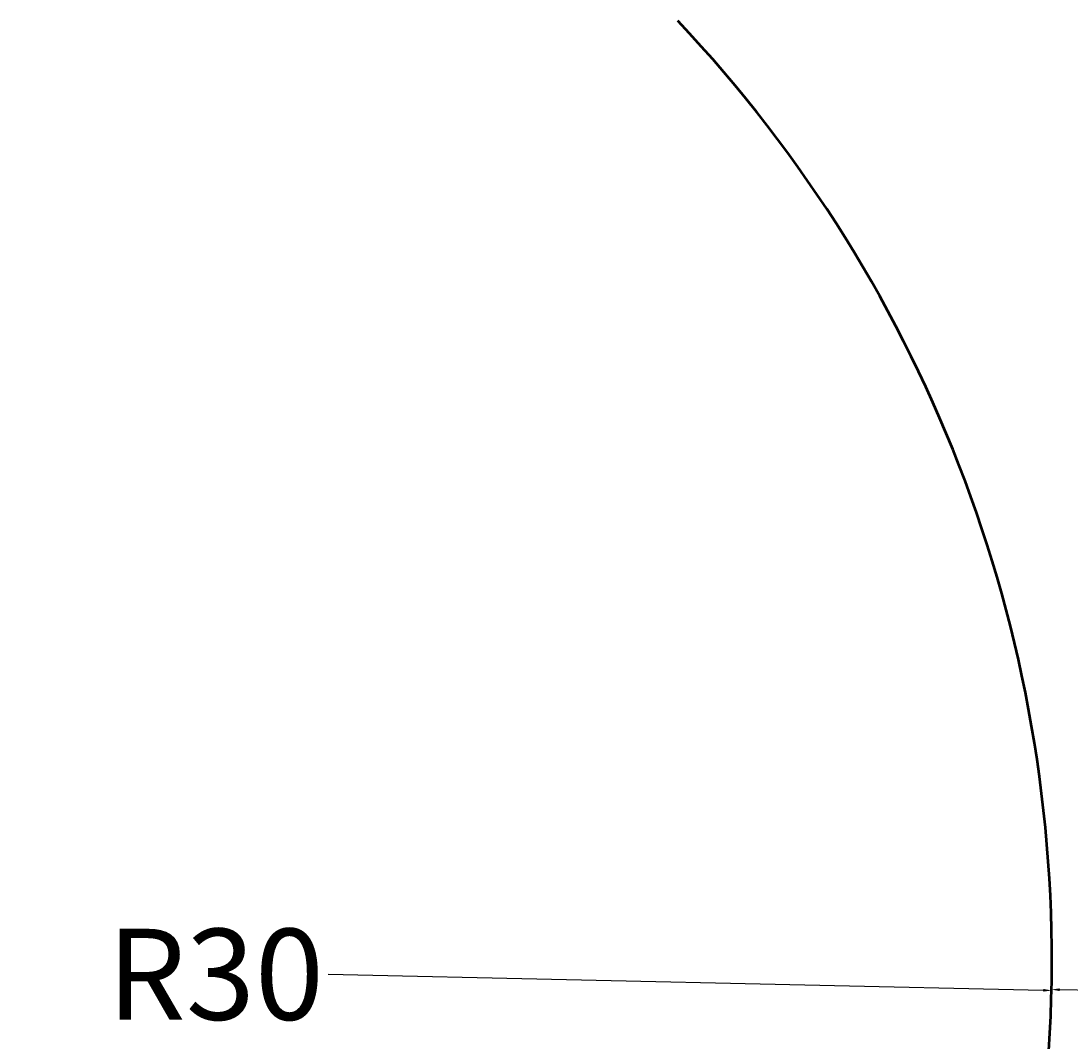
# Model space of a CAD drawing. Units: millimetres. Extents: x -60 to 113, y -37 to 126.
# Tile 8 of 17: x -23 to 0, y 48 to 70. Entities that reach past the tile are written whole.
import ezdxf

# ---------------------------------------------------------------- set-up
doc = ezdxf.new("R2010")
doc.units = ezdxf.units.MM
doc.header["$MEASUREMENT"] = 0
doc.layers.add('M-DIMS', color=2, linetype='Continuous', lineweight=25)
doc.layers.add('M-OUTL', color=7, linetype='Continuous', lineweight=50)
doc.styles.get("Standard").update_dxf_attribs({"font": 'arial.ttf'})
doc.dimstyles.get("Standard").update_dxf_attribs({"dimtxt": 0.18, "dimasz": 0.18, "dimexe": 0.18, "dimexo": 0.0625, "dimgap": 0.09, "dimtad": 0, "dimtih": 1, "dimtoh": 1, "dimdec": 4, "dimzin": 0, "dimdsep": 46, "dimtxsty": 'Standard', "dimcen": 0.09, "dimadec": 0, "dimazin": 0, "dimtfac": 1, "dimtdec": 4, "dimtofl": 0, "dimtmove": 0, "dimatfit": 3, "dimfxl": 1, "dimtolj": 1, "dimtzin": 0, "dimarcsym": 0})

# ---------------------------------------------------------------- blocks, each defined once
blk = doc.blocks.new('*D6')
at = {"layer": 'Defpoints', "color": 0, "transparency": 16777216}
for p in [(-30.775, 49.351), (-0.783, 48.68)]:
    blk.add_point(p, dxfattribs=at)
at = {"layer": 'M-DIMS', "color": 0, "lineweight": -2, "transparency": 16777216}
blk.add_line((-16.661, 49.035), (-0.963, 48.684), dxfattribs=at)
at = {"layer": 'M-DIMS', "color": 0, "transparency": 16777216}
blk.add_solid([(-0.962, 48.714), (-0.963, 48.654), (-0.783, 48.68)], dxfattribs=at)
at = {"layer": 'M-DIMS', "color": 0, "transparency": 16777216, "insert": (-19.137, 49.035), "char_height": 0.18, "attachment_point": 5}
blk.add_mtext('\\A1;{\\H11.11111x;R30}', dxfattribs=at)
blk = doc.blocks.new('*D7')
at = {"layer": 'Defpoints', "color": 0, "transparency": 16777216}
for p in [(48.606, 76.822), (-30.775, 49.351)]:
    blk.add_point(p, dxfattribs=at)
at = {"layer": 'M-DIMS', "color": 0, "lineweight": -2, "transparency": 16777216}
for p, q in [((37.821, 73.09), (48.435, 76.764)), ((37.641, 73.09), (37.821, 73.09))]:
    blk.add_line(p, q, dxfattribs=at)
at = {"layer": 'M-DIMS', "color": 0, "transparency": 16777216}
blk.add_solid([(48.426, 76.792), (48.445, 76.735), (48.606, 76.822)], dxfattribs=at)
at = {"layer": 'M-DIMS', "color": 0, "transparency": 16777216, "insert": (35.165, 73.09), "char_height": 0.18, "attachment_point": 5}
blk.add_mtext('\\A1;{\\H11.11111x;R84}', dxfattribs=at)
blk = doc.blocks.new('*D12')
at = {"layer": 'Defpoints', "color": 0, "transparency": 16777216}
for p in [(10.532, 88.533), (-58.719, 6.903), (11.329, 6.903)]:
    blk.add_point(p, dxfattribs=at)
at = {"layer": 'M-DIMS', "color": 0, "lineweight": -2, "transparency": 16777216}
for p, q in [((10.47, 88.533), (-58.899, 88.533)), ((-58.719, 88.353), (-58.719, 48.829)), ((-58.719, 7.083), (-58.719, 46.607)), ((11.267, 6.903), (-58.899, 6.903))]:
    blk.add_line(p, q, dxfattribs=at)
at = {"layer": 'M-DIMS', "color": 0, "transparency": 16777216}
for points in [[(-58.749, 88.353), (-58.689, 88.353), (-58.719, 88.533)], [(-58.749, 7.083), (-58.689, 7.083), (-58.719, 6.903)]]:
    blk.add_solid(points, dxfattribs=at)
at = {"layer": 'M-DIMS', "color": 0, "transparency": 16777216, "insert": (-58.719, 47.718), "char_height": 0.18, "attachment_point": 5}
blk.add_mtext('\\A1;{\\H11.11111x;82}', dxfattribs=at)
blk = doc.blocks.new('*D24')
at = {"layer": 'Defpoints', "color": 0, "transparency": 16777216}
for p in [(48.596, 76.851), (-30.775, 49.351)]:
    blk.add_point(p, dxfattribs=at)
at = {"layer": 'M-DIMS', "color": 0, "lineweight": -2, "transparency": 16777216}
for p, q in [((96.218, 93.35), (48.766, 76.909)), ((96.398, 93.35), (96.218, 93.35)), ((-30.865, 49.351), (-30.685, 49.351)), ((-30.775, 49.261), (-30.775, 49.441))]:
    blk.add_line(p, q, dxfattribs=at)
at = {"layer": 'M-DIMS', "color": 0, "transparency": 16777216}
blk.add_solid([(48.756, 76.938), (48.776, 76.881), (48.596, 76.851)], dxfattribs=at)
at = {"layer": 'M-DIMS', "color": 0, "transparency": 16777216, "insert": (97.018, 93.35), "char_height": 0.18, "attachment_point": 5}
blk.add_mtext('\\A1;R84.0000', dxfattribs=at)
blk = doc.blocks.new('*D25')
at = {"layer": 'Defpoints', "color": 0, "transparency": 16777216}
for p in [(-30.775, 49.351), (-0.782, 48.7)]:
    blk.add_point(p, dxfattribs=at)
at = {"layer": 'M-DIMS', "color": 0, "lineweight": -2, "transparency": 16777216}
for p, q in [((-30.865, 49.351), (-30.685, 49.351)), ((-30.775, 49.261), (-30.775, 49.441)), ((17.214, 48.309), (-0.602, 48.696))]:
    blk.add_line(p, q, dxfattribs=at)
at = {"layer": 'M-DIMS', "color": 0, "transparency": 16777216}
blk.add_solid([(-0.602, 48.726), (-0.603, 48.666), (-0.782, 48.7)], dxfattribs=at)
at = {"layer": 'M-DIMS', "color": 0, "transparency": 16777216, "insert": (17.833, 48.309), "char_height": 0.18, "attachment_point": 5}
blk.add_mtext('\\A1;R30.0000', dxfattribs=at)

msp = doc.modelspace()

# ---------------------------------------------------------------- linework, layer by layer
at = {"layer": 'M-OUTL'}
msp.add_arc((-30.77517, 49.3506), 30, 311.866655, 43.425324, dxfattribs=at)

# ---------------------------------------------------------------- dimensions: what is measured, and where the dimension line sits
at = {"layer": 'M-DIMS'}
for mpoint, picture, middle in [((48.59582, 76.85052), '*D24', (97.01779, 93.35047)), ((-0.78224, 48.69961), '*D25', (17.21352, 48.30902))]:
    dim = msp.add_radius_dim(center=(-30.77517, 49.3506), mpoint=mpoint, dimstyle='Standard', override={"dimdec": 4, "dimlfac": 1, "dimrnd": 0, "dimzin": 0, "dimdsep": 46, "dimlunit": 2}, dxfattribs=at)
    dim.commit()
    dim.dimension.update_dxf_attribs({"geometry": picture, "text_midpoint": middle, "dimtype": 164})
dim = msp.add_linear_dim(base=(-58.71857, 6.9027), p1=(10.53227, 88.53289), p2=(11.32938, 6.9027), angle=90, text='{\\H11.11111x;82}', dimstyle='Standard', override={"dimclrd": 0, "dimclre": 0, "dimclrt": 0}, dxfattribs=at)
dim.commit()
dim.dimension.update_dxf_attribs({"geometry": '*D12', "text_midpoint": (-58.71857, 47.71779)})
for mpoint, text, picture, middle in [((48.60556, 76.82239), '{\\H11.11111x;R84}', '*D7', (35.16548, 73.09007)), ((-0.78268, 48.6796), '{\\H11.11111x;R30}', '*D6', (-16.66078, 49.03483))]:
    dim = msp.add_radius_dim(center=(-30.77517, 49.3506), mpoint=mpoint, text=text, dimstyle='Standard', override={"dimclrd": 0, "dimclre": 0, "dimclrt": 0}, dxfattribs=at)
    dim.commit()
    dim.dimension.update_dxf_attribs({"geometry": picture, "text_midpoint": middle, "dimtype": 164})

doc.saveas('drawing.dxf')
